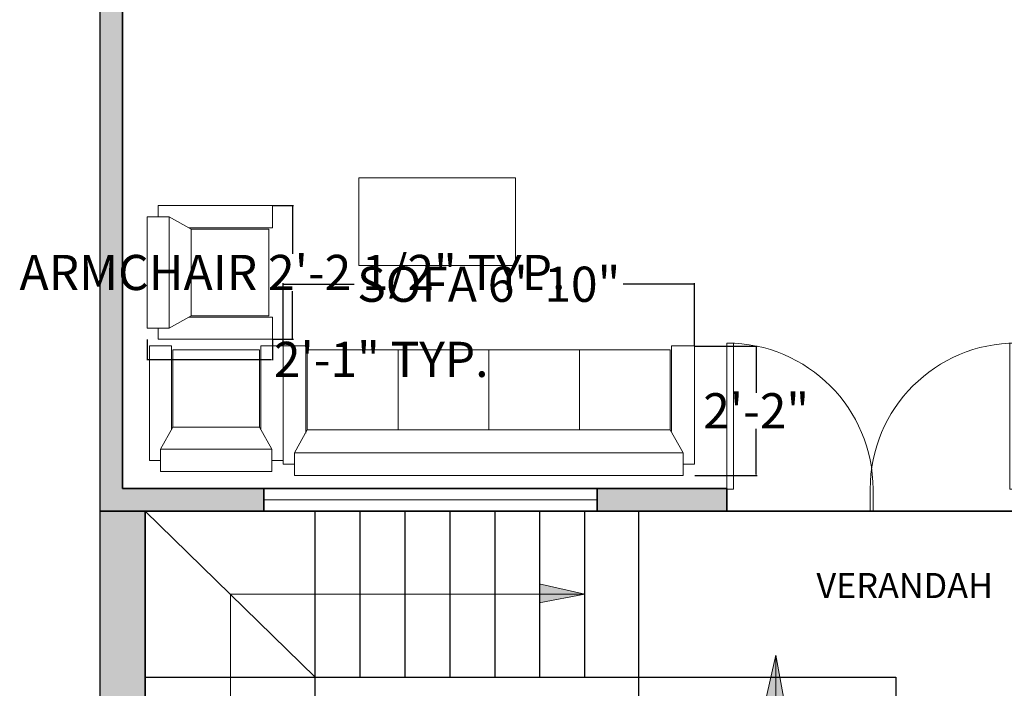
# Model space of a CAD drawing. Units: inches. Extents: x 0 to 4258, y 0 to 3769.
# Tile 16 of 30: x 3663 to 3859, y 3128 to 3261. Entities that reach past the tile are written whole.
import ezdxf

# ---------------------------------------------------------------- set-up
doc = ezdxf.new("R2010")
doc.units = ezdxf.units.IN
doc.header["$MEASUREMENT"] = 0
doc.layers.get('0').update_dxf_attribs({"color": 16})
for name, color, linetype, lineweight in [('A-ANNO-DIMS', 250, 'Continuous', 18), ('A-ANNO-SYMB', 250, 'Continuous', 18), ('A-AREA-IDEN', 250, 'Continuous', 18), ('A-FLOR-STRS', 150, 'Continuous', 25), ('A-WALL-PATT', 16, 'Continuous', 13), ('C-PROP', 150, 'Continuous', 25), ('doors', 250, 'Continuous', 18), ('furniture', 13, 'Continuous', 18), ('walls', 251, 'Continuous', 35), ('windows', 121, 'Continuous', 18)]:
    doc.layers.add(name, color=color, linetype=linetype, lineweight=lineweight)
doc.styles.get("Standard").update_dxf_attribs({"font": 'arial.ttf'})
doc.dimstyles.get("Standard").update_dxf_attribs({"dimtxt": 7, "dimasz": 0.18, "dimexe": 0.18, "dimexo": 0.0625, "dimgap": 0.09, "dimtad": 0, "dimtih": 1, "dimtoh": 1, "dimzin": 0, "dimdsep": 46, "dimlunit": 3, "dimtxsty": 'Standard', "dimcen": 0.09, "dimadec": 0, "dimazin": 0, "dimtfac": 1, "dimtofl": 0, "dimtmove": 0, "dimatfit": 3, "dimfxl": 1, "dimtolj": 1, "dimtzin": 0, "dimarcsym": 0})

# ---------------------------------------------------------------- blocks, each defined once
blk = doc.blocks.new('FABRIC SOFA 1S')
at = {"layer": 'furniture'}
for p, q in [((3, 18.12), (34, 18.12)), ((3, 15.12), (3, 18.12)), ((34, 12.12), (34, 18.12)), ((0, -15.12), (0, 15.12)), ((6, 15.12), (0, 15.12)), ((6, -15.12), (6, 15.12)), ((12, 11.75), (6, 15.12)), ((11.33, 12.12), (34, 12.12)), ((6, -15.12), (12, -11.75)), ((11.33, -12.12), (34, -12.12)), ((34, -12.12), (34, -18.12)), ((6, -15.12), (0, -15.12)), ((3, -18.12), (3, -15.12)), ((3, -18.12), (34, -18.12))]:
    blk.add_line(p, q, dxfattribs=at)
blk.add_lwpolyline([(12, -11.75), (12, 11.75), (33, 11.75), (33, -11.75)], close=True, dxfattribs=at)
blk = doc.blocks.new('FABRIC SOFA 4S')
at = {"layer": 'furniture'}
for p, q in [((3, 54), (34, 54)), ((3, 51), (3, 54)), ((34, 48), (34, 54)), ((0, -51), (0, 51)), ((6, 51), (0, 51)), ((6, -51), (6, 51)), ((12, 47.63), (6, 51)), ((11.14, 48), (34, 48)), ((33, 23.81), (12, 23.81)), ((33, 0), (12, 0)), ((33, -23.81), (12, -23.81)), ((6, -51), (12, -47.63)), ((11.54, -48), (34, -48)), ((34, -48), (34, -54)), ((6, -51), (0, -51)), ((3, -54), (3, -51)), ((3, -54), (34, -54))]:
    blk.add_line(p, q, dxfattribs=at)
blk.add_lwpolyline([(12, -47.63), (12, 47.63), (33, 47.63), (33, -47.63)], close=True, dxfattribs=at)
blk = doc.blocks.new('*U23')
for p, q in [((0, 0), (0, -6)), ((40, 0), (40, -6))]:
    blk.add_line(p, q)
blk.add_lwpolyline([(0, 0), (0, 40), (1.75, 40), (1.75, 0)], close=True)
blk.add_arc((0, 0), 40, 0, 90)
blk = doc.blocks.new('STAIR-DIRECTION-ARROW')
h = blk.add_hatch(color=256)
h.dxf.hatch_style = 1
h.paths.add_polyline_path([(14.74, 3.76), (14.74, 1.69), (23.85, 1.69)])
h.paths.add_polyline_path([(23.85, 1.69), (14.74, 1.69), (14.74, 0)])
for p, q in [((23.85, 1.69), (14.74, 3.76)), ((0, 1.69), (23.85, 1.69)), ((14.74, 0), (23.85, 1.69))]:
    blk.add_line(p, q)
blk = doc.blocks.new('*D46')
at = {"layer": 'A-ANNO-DIMS', "color": 0, "lineweight": -2, "transparency": 16777216}
for p, q in [((3715.25, 3196.22), (3715.25, 3208.63)), ((3715.43, 3208.45), (3729.43, 3208.45)), ((3796.97, 3208.45), (3782.97, 3208.45)), ((3797.15, 3196.22), (3797.15, 3208.63))]:
    blk.add_line(p, q, dxfattribs=at)
at = {"layer": 'A-ANNO-DIMS', "color": 0, "transparency": 16777216}
for points in [[(3715.43, 3208.48), (3715.43, 3208.42), (3715.25, 3208.45)], [(3796.97, 3208.48), (3796.97, 3208.42), (3797.15, 3208.45)]]:
    blk.add_solid(points, dxfattribs=at)
at = {"layer": 'Defpoints', "color": 0, "transparency": 16777216}
for p in [(3715.25, 3208.45), (3715.25, 3196.16), (3797.15, 3196.16)]:
    blk.add_point(p, dxfattribs=at)
at = {"layer": 'A-ANNO-DIMS', "color": 0, "transparency": 16777216, "insert": (3756.2, 3208.45), "char_height": 7, "attachment_point": 5}
blk.add_mtext('\\A1;SOFA 6\'-10"', dxfattribs=at)
blk = doc.blocks.new('*D47')
at = {"layer": 'A-ANNO-DIMS', "color": 0, "lineweight": -2, "transparency": 16777216}
for p, q in [((3797.21, 3196.16), (3809.62, 3196.16)), ((3809.44, 3195.98), (3809.44, 3186.87)), ((3809.44, 3170.56), (3809.44, 3179.67)), ((3797.21, 3170.38), (3809.62, 3170.38))]:
    blk.add_line(p, q, dxfattribs=at)
at = {"layer": 'A-ANNO-DIMS', "color": 0, "transparency": 16777216}
for points in [[(3809.41, 3195.98), (3809.47, 3195.98), (3809.44, 3196.16)], [(3809.41, 3170.56), (3809.47, 3170.56), (3809.44, 3170.38)]]:
    blk.add_solid(points, dxfattribs=at)
at = {"layer": 'Defpoints', "color": 0, "transparency": 16777216}
for p in [(3797.15, 3196.16), (3809.44, 3196.16), (3797.15, 3170.38)]:
    blk.add_point(p, dxfattribs=at)
at = {"layer": 'A-ANNO-DIMS', "color": 0, "transparency": 16777216, "insert": (3809.44, 3183.27), "char_height": 7, "attachment_point": 5}
blk.add_mtext('\\A1;2\'-2"', dxfattribs=at)
blk = doc.blocks.new('*D50')
at = {"layer": 'A-ANNO-DIMS', "color": 0, "lineweight": -2, "transparency": 16777216}
for p, q in [((3713.19, 3224.1), (3717.3, 3224.1)), ((3717.12, 3223.92), (3717.12, 3214.5)), ((3717.12, 3197.67), (3717.12, 3207.08)), ((3713.19, 3197.49), (3717.3, 3197.49))]:
    blk.add_line(p, q, dxfattribs=at)
at = {"layer": 'A-ANNO-DIMS', "color": 0, "transparency": 16777216}
for points in [[(3717.09, 3223.92), (3717.15, 3223.92), (3717.12, 3224.1)], [(3717.09, 3197.67), (3717.15, 3197.67), (3717.12, 3197.49)]]:
    blk.add_solid(points, dxfattribs=at)
at = {"layer": 'Defpoints', "color": 0, "transparency": 16777216}
for p in [(3713.13, 3224.1), (3717.12, 3224.1), (3713.13, 3197.49)]:
    blk.add_point(p, dxfattribs=at)
at = {"layer": 'A-ANNO-DIMS', "color": 0, "transparency": 16777216, "insert": (3717.12, 3210.79), "char_height": 7, "attachment_point": 5}
blk.add_mtext('\\A1;ARMCHAIR 2\'-2 1/2" TYP.', dxfattribs=at)
blk = doc.blocks.new('*D51')
at = {"layer": 'A-ANNO-DIMS', "color": 0, "lineweight": -2, "transparency": 16777216}
for p, q in [((3688.17, 3197.43), (3688.17, 3193.32)), ((3713.13, 3197.43), (3713.13, 3193.32)), ((3688.35, 3193.5), (3712.95, 3193.5)), ((3713.13, 3193.5), (3713.31, 3193.5))]:
    blk.add_line(p, q, dxfattribs=at)
at = {"layer": 'A-ANNO-DIMS', "color": 0, "transparency": 16777216}
for points in [[(3688.35, 3193.53), (3688.35, 3193.47), (3688.17, 3193.5)], [(3712.95, 3193.53), (3712.95, 3193.47), (3713.13, 3193.5)]]:
    blk.add_solid(points, dxfattribs=at)
at = {"layer": 'Defpoints', "color": 0, "transparency": 16777216}
for p in [(3688.17, 3197.49), (3713.13, 3197.49), (3713.13, 3193.5)]:
    blk.add_point(p, dxfattribs=at)
at = {"layer": 'A-ANNO-DIMS', "color": 0, "transparency": 16777216, "insert": (3734.79, 3193.5), "char_height": 7, "attachment_point": 5}
blk.add_mtext('\\A1;2\'-1" TYP.', dxfattribs=at)

msp = doc.modelspace()

# ---------------------------------------------------------------- hatches: boundary and pattern name
at = {"layer": 'A-WALL-PATT'}
h = msp.add_hatch(color=256, dxfattribs=at)
h.dxf.hatch_style = 1
h.paths.add_polyline_path([(3753.804, 3425.793), (3753.804, 3437.642), (3815.304, 3437.642), (3815.304, 3421.293), (3819.804, 3421.293), (3819.804, 3442.142), (3749.304, 3442.142), (3749.304, 3425.793), (3683.304, 3425.793), (3683.304, 3652.293), (3773.304, 3652.293), (3773.304, 3638.769), (3777.804, 3638.769), (3777.804, 3656.793), (3678.804, 3656.793), (3678.804, 3163.293), (3711.393, 3163.293), (3711.393, 3167.793), (3683.304, 3167.793), (3683.304, 3374.793), (3693.303, 3374.793), (3693.303, 3379.293), (3683.304, 3379.293), (3683.304, 3421.293), (3749.304, 3421.293), (3749.304, 3379.293), (3741.449, 3379.293), (3741.449, 3374.793), (3753.804, 3374.793)])
h = msp.add_hatch(color=256, dxfattribs=at)
h.dxf.hatch_style = 1
h.paths.add_polyline_path([(3687.804, 3163.293), (3678.804, 3163.293), (3678.804, 2995.293), (3687.804, 2995.293)])
h.paths.add_polyline_path([(3973.039, 3461.793), (3866.304, 3461.793), (3866.304, 3457.293), (3973.039, 3457.293)])
h.paths.add_polyline_path([(4034.304, 3461.793), (4016.474, 3461.793), (4016.474, 3457.293), (4034.304, 3457.293)])
h = msp.add_hatch(color=256, dxfattribs=at)
h.dxf.hatch_style = 1
h.paths.add_polyline_path([(3803.626, 3167.657), (3803.626, 3167.793), (3777.808, 3167.793), (3777.808, 3163.293), (3803.626, 3163.293)])
h = msp.add_hatch(color=256, dxfattribs=at)
h.dxf.hatch_style = 1
h.paths.add_polyline_path([(3803.626, 3167.657), (3803.626, 3167.793), (3777.808, 3167.793), (3777.808, 3163.293), (3803.626, 3163.293)])
h = msp.add_hatch(color=256, dxfattribs=at)
h.dxf.hatch_style = 1
h.paths.add_polyline_path([(3803.626, 3167.657), (3803.626, 3167.793), (3777.808, 3167.793), (3777.808, 3163.293), (3803.626, 3163.293)])

# ---------------------------------------------------------------- linework, layer by layer
at = {"layer": 'A-ANNO-SYMB'}
for p, q in [((3751.481, 3146.777), (3704.8, 3146.777)), ((3704.8, 3146.777), (3704.8, 3018.327)), ((3813.379, 3130.262), (3813.379, 3110.595))]:
    msp.add_line(p, q, dxfattribs=at)
at = {"layer": 'A-FLOR-STRS'}
for p, q in [((3721.668, 3130.262), (3687.804, 3163.293)), ((3721.668, 3028.53), (3721.668, 3163.293)), ((3730.612, 3130.262), (3730.612, 3163.293)), ((3739.556, 3130.262), (3739.556, 3163.293)), ((3748.501, 3130.262), (3748.501, 3163.293)), ((3757.445, 3130.262), (3757.445, 3163.293)), ((3766.389, 3130.262), (3766.389, 3163.293)), ((3775.334, 3130.262), (3775.334, 3163.293)), ((3786.102, 3122.34), (3786.102, 3163.293)), ((3687.804, 3130.262), (3721.668, 3130.262)), ((3721.668, 3130.262), (3837.232, 3130.262)), ((3837.232, 3130.262), (3837.232, 3075.983))]:
    msp.add_line(p, q, dxfattribs=at)
at = {"layer": 'C-PROP'}
msp.add_line((3678.804, 2995.293), (3678.804, 3656.793), dxfattribs=at)
at = {"layer": 'furniture'}
for p, q in [((3761.535, 3229.65), (3730.363, 3229.65)), ((3730.363, 3229.65), (3730.363, 3212.174)), ((3761.535, 3212.174), (3761.535, 3229.65)), ((3730.363, 3212.174), (3761.535, 3212.174))]:
    msp.add_line(p, q, dxfattribs=at)
at = {"layer": 'walls'}
for p, q in [((3683.304, 3167.793), (3683.304, 3374.793)), ((3683.304, 3167.793), (3803.626, 3167.793)), ((3711.393, 3167.793), (3711.393, 3163.293)), ((3777.808, 3163.293), (3777.808, 3167.793)), ((3803.626, 3167.793), (3803.626, 3163.293)), ((3678.804, 3163.293), (3861.804, 3163.293)), ((3687.804, 2995.293), (3687.804, 3163.293))]:
    msp.add_line(p, q, dxfattribs=at)
at = {"layer": 'windows'}
for p, q in [((3777.808, 3167.793), (3711.393, 3167.793)), ((3711.393, 3165.543), (3777.808, 3165.543)), ((3711.393, 3163.293), (3777.808, 3163.293))]:
    msp.add_line(p, q, dxfattribs=at)

# ---------------------------------------------------------------- block references
at = {"layer": 'A-ANNO-SYMB'}
msp.add_blockref('STAIR-DIRECTION-ARROW', (3751.481, 3145.086), dxfattribs=at)
at = {"layer": 'A-ANNO-SYMB', "rotation": 90.00000000000003}
msp.add_blockref('STAIR-DIRECTION-ARROW', (3815.049, 3110.82), dxfattribs=at)
at = {"layer": 'doors', "yscale": 0.7272131312874193, "zscale": 0.7272131312874193}
for p, xscale in [((3803.626, 3167.657), 0.7272131312874193), ((3861.23, 3167.657), -0.7272131312874193)]:
    msp.add_blockref('*U23', p, dxfattribs=dict(at, xscale=xscale))
at = {"layer": 'furniture', "xscale": 0.7339463821036302, "yscale": 0.7339463821036302, "zscale": 0.7339463821036302}
msp.add_blockref('FABRIC SOFA 1S', (3688.173, 3210.793), dxfattribs=at)
at = {"layer": 'furniture'}
for name, p, xscale, yscale, zscale, rotation in [('FABRIC SOFA 1S', (3701.943, 3171.208), 0.7339463821036302, 0.7339463821036302, 0.7339463821036302, 90.00000000000087), ('FABRIC SOFA 4S', (3756.198, 3170.377), 0.7583822975527559, 0.7583822975527559, 0.7583822975527559, 89.99999999999999)]:
    msp.add_blockref(name, p, dxfattribs=dict(at, xscale=xscale, yscale=yscale, zscale=zscale, rotation=rotation))

# ---------------------------------------------------------------- texts
at = {"layer": 'A-AREA-IDEN'}
msp.add_text('VERANDAH', height=5, dxfattribs=at).set_placement((3821.436, 3145.999))

# ---------------------------------------------------------------- dimensions: what is measured, and where the dimension line sits
at = {"layer": 'A-ANNO-DIMS'}
for base, p1, p2, angle, text, picture, middle in [((3717.118, 3224.096), (3713.127, 3197.49), (3713.127, 3224.096), 90, 'ARMCHAIR <> TYP.', '*D50', (3717.118, 3210.793)), ((3715.245, 3208.448), (3797.151, 3196.162), (3715.245, 3196.162), 180, 'SOFA <>', '*D46', (3756.198, 3208.448))]:
    dim = msp.add_linear_dim(base=base, p1=p1, p2=p2, angle=angle, text=text, dimstyle='Standard', override={"dimdec": 1, "dimlfac": 1, "dimrnd": 0, "dimzin": 1, "dimdsep": 46, "dimlunit": 4, "dimfrac": 2}, dxfattribs=at)
    dim.commit()
    dim.dimension.update_dxf_attribs({"geometry": picture, "text_midpoint": middle})
dim = msp.add_linear_dim(base=(3713.127, 3193.5), p1=(3688.173, 3197.49), p2=(3713.127, 3197.49), text='<> TYP.', dimstyle='Standard', override={"dimdec": 1, "dimlfac": 1, "dimrnd": 0, "dimzin": 1, "dimdsep": 46, "dimlunit": 4, "dimfrac": 2}, dxfattribs=at)
dim.commit()
dim.dimension.update_dxf_attribs({"geometry": '*D51', "text_midpoint": (3734.791, 3193.5)})
dim = msp.add_linear_dim(base=(3809.436, 3196.162), p1=(3797.151, 3170.377), p2=(3797.151, 3196.162), angle=90, dimstyle='Standard', override={"dimdec": 1, "dimlfac": 1, "dimrnd": 0, "dimzin": 1, "dimdsep": 46, "dimlunit": 4, "dimfrac": 2}, dxfattribs=at)
dim.commit()
dim.dimension.update_dxf_attribs({"geometry": '*D47', "text_midpoint": (3809.436, 3183.27)})

doc.saveas('drawing.dxf')
